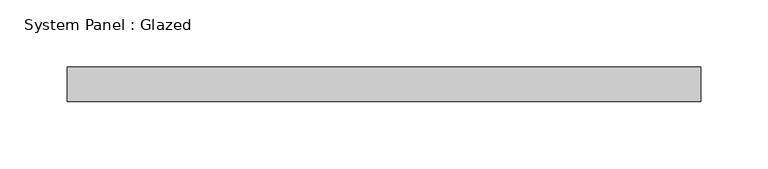
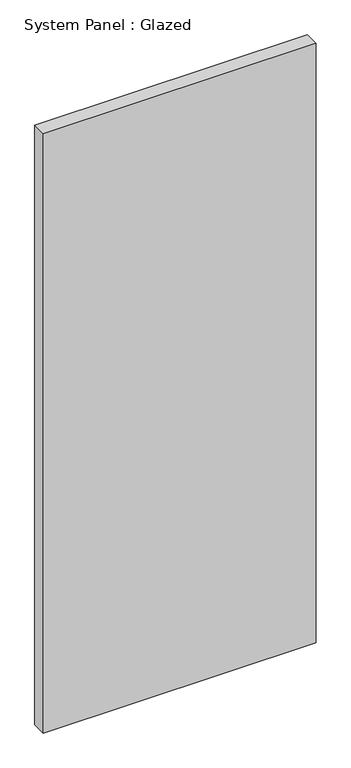
"""IFC4 building model written with IfcOpenShell, lengths in millimetres: plate geometry, System Panel : Glazed."""

from ifc_helpers import new_model, si_unit, origin, origin_with_axes, place, context, project, spatial, polyline, outline, extrude, source, transform, mapped, element, save


def system_panel_glazed_90898af3(model_context):
    return source(origin(), model_context, "Body", "SweptSolid", [
        extrude(outline(polyline([(234.9892031, 19.05), (-234.9892031, 19.05), (-234.9892031, 44.45), (234.9892031, 44.45), (234.9892031, 19.05)])), origin_with_axes(), (0.0, 0.0, 1.0), 1092.2),
    ])


if __name__ == "__main__":
    model = new_model("IFC4")
    model_context = context("Model", 3, world=origin())
    ifc_project = project(units=[si_unit("LENGTHUNIT", "METRE", prefix="MILLI")], contexts=[model_context])
    site = spatial("IfcSite", under=ifc_project)
    building = spatial("IfcBuilding", under=site)
    placement = place(None, origin())
    system_panel_glazed_shape = system_panel_glazed_90898af3(model_context)
    element("IfcPlate", 1, ObjectType="System Panel : Glazed", at=placement, inside=building, context=model_context, shape_type="MappedRepresentation", body=[
        mapped(system_panel_glazed_shape, transform((0.0, 0.0, 0.0), x_axis=(1.0, 0.0, 0.0), y_axis=(0.0, 1.0, 0.0), z_axis=(0.0, 0.0, 1.0))),
    ])
    save(model, "model.ifc")

# Revit data of these elements
# Type "System Panel : Glazed"
#   Construction Type Id = "GSP4R"
#   Analytic Construction = "1/8 in Pilkington single glazing"
#   Visual Light Transmittance = 0.9
#   Solar Heat Gain Coefficient = 0.86
#   Heat Transfer Coefficient (U) = 1.18115 BTU/(h·ft²·°F)
#   Define Thermal Properties by = 1
# Element 1 (IfcPlate, "System Panel : Glazed")
#   Materials on its faces: "Glass"
# Materials
#   "Glass": class "Glass", colour RGB 0 128 192, transparency 0.75, Description = "Soda Lime Glass", Cost = 0
